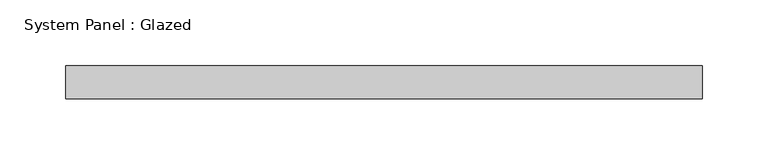
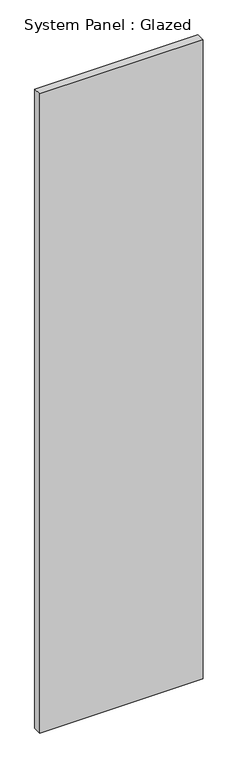
"""IFC4 building model written with IfcOpenShell, lengths in millimetres: plate geometry, System Panel : Glazed."""

from ifc_helpers import new_model, si_unit, origin, origin_with_axes, place, context, project, spatial, polyline, outline, extrude, source, transform, mapped, element, save


def system_panel_glazed_1490133a(model_context):
    return source(origin(), model_context, "Body", "SweptSolid", [
        extrude(outline(polyline([(242.9071378, 19.05), (-242.9071378, 19.05), (-242.9071378, 44.45), (242.9071378, 44.45), (242.9071378, 19.05)])), origin_with_axes(), (0.0, 0.0, 1.0), 2006.6),
    ])


if __name__ == "__main__":
    model = new_model("IFC4")
    model_context = context("Model", 3, world=origin())
    ifc_project = project(units=[si_unit("LENGTHUNIT", "METRE", prefix="MILLI")], contexts=[model_context])
    site = spatial("IfcSite", under=ifc_project)
    building = spatial("IfcBuilding", under=site)
    placement = place(None, origin())
    system_panel_glazed_shape = system_panel_glazed_1490133a(model_context)
    element("IfcPlate", 1, ObjectType="System Panel : Glazed", at=placement, inside=building, context=model_context, shape_type="MappedRepresentation", body=[
        mapped(system_panel_glazed_shape, transform((0.0, 0.0, 0.0), x_axis=(1.0, 0.0, 0.0), y_axis=(0.0, 1.0, 0.0), z_axis=(0.0, 0.0, 1.0))),
    ])
    save(model, "model.ifc")

# Revit data of these elements
# Type "System Panel : Glazed"
#   Construction Type Id = "GSP4R"
#   Analytic Construction = "1/8 in Pilkington single glazing"
#   Visual Light Transmittance = 0.9
#   Solar Heat Gain Coefficient = 0.86
#   Heat Transfer Coefficient (U) = 1.18115 BTU/(h·ft²·°F)
#   Define Thermal Properties by = 1
# Element 1 (IfcPlate, "System Panel : Glazed")
#   Materials on its faces: "Glass"
# Materials
#   "Glass": class "Glass", colour RGB 0 128 192, transparency 0.75, Description = "Soda Lime Glass", Cost = 0
